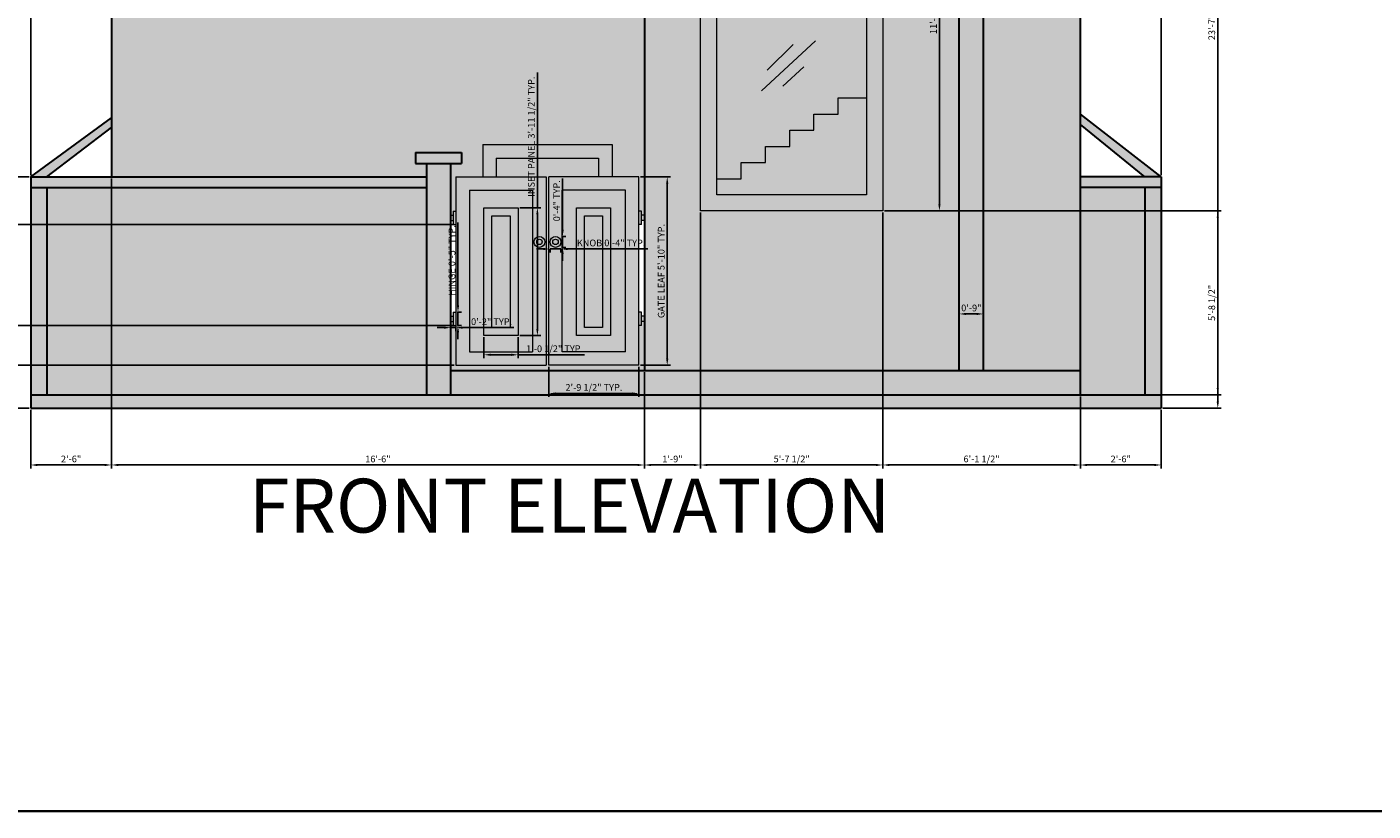
# Model space of a CAD drawing. Units: inches. Extents: x 6038 to 7543, y 3772 to 5131.
# Tile 2 of 14: x 6290 to 6790, y 3772 to 4063. Entities that reach past the tile are written whole.
import ezdxf

# ---------------------------------------------------------------- set-up
doc = ezdxf.new("R2010")
doc.units = ezdxf.units.IN
for name, color, linetype, lineweight in [('A-ANNO-DIMS', 4, 'Continuous', 18), ('A-ANNO-TITL', 3, 'Continuous', 30), ('A-ANNO-TTLB', 1, 'Continuous', 35), ('A-ELEV', 7, 'Continuous', 30), ('A-ELEV-DOOR-PATT', 209, 'Continuous', 13), ('A-ELEV-FRAM-PATT', 7, 'Continuous', 13), ('A-ELEV-GATE', 7, 'Continuous', 20), ('A-ELEV-GLAZ', 7, 'Continuous', 18), ('A-ELEV-STRS', 7, 'Continuous', 18)]:
    doc.layers.add(name, color=color, linetype=linetype, lineweight=lineweight)
for name, color, linetype, lineweight, true_color in [('A-ELEV-BASE-PATT', 253, 'Continuous', 13, 0xb4b5b6), ('A-ELEV-GLAZ-PATT', 141, 'Continuous', 13, 0xadddf7), ('A-ELEV-METL-PATT', 252, 'Continuous', 13, 0x939598), ('A-ELEV-PANL-PATT', 165, 'Continuous', 13, 0x5e67af), ('A-ELEV-TRIM-PATT', 85, 'Continuous', 13, 0x58ba48), ('A-ELEV-WALL-PATT', 11, 'Continuous', 13, 0xf27172)]:
    doc.layers.add(name, color=color, linetype=linetype, lineweight=lineweight, true_color=true_color)
doc.styles.get("Standard").update_dxf_attribs({"font": 'arial.ttf'})
doc.dimstyles.new('ISO-25', dxfattribs={"dimtxt": 2.5, "dimasz": 2.5, "dimexe": 1.25, "dimexo": 0.625, "dimtad": 1, "dimdec": 0, "dimlunit": 3, "dimtxsty": 'Standard', "dimcen": 2.5, "dimadec": 0, "dimazin": 0, "dimtfac": 1, "dimtdec": 0, "dimtmove": 0, "dimatfit": 3, "dimfxl": 1, "dimarcsym": 0})

# ---------------------------------------------------------------- blocks, each defined once
blk = doc.blocks.new('GATE-LEAF-FRAME-ELEV')
for p, q in [((0, 70), (0, 0)), ((0, 70), (33.5, 70)), ((33.5, 70), (33.5, 0)), ((5, 65), (5, 5)), ((5, 65), (28.5, 65)), ((28.5, 65), (28.5, 5)), ((5, 5), (28.5, 5)), ((0, 0), (33.5, 0))]:
    blk.add_line(p, q)
blk = doc.blocks.new('GATE-LEAF-INSET-ELEV')
for points in [[(0, 47.53), (12.73, 47.53), (12.73, 0), (0, 0)], [(3, 44.53), (9.73, 44.53), (9.73, 3), (3, 3)]]:
    blk.add_lwpolyline(points, close=True)
blk = doc.blocks.new('GATE-HINGE-ELEV')
for p, q in [((0, 3.5), (1, 3.5)), ((0, 1.5), (1, 1.5)), ((1, 5), (2, 5)), ((1, 5), (1, 0)), ((1, 0), (2, 0))]:
    blk.add_line(p, q)
blk = doc.blocks.new('GATE-KNOB-ELEV')
for radius in [2.03, 1.03]:
    blk.add_circle((2.03, 2.03), radius)
blk = doc.blocks.new('GLASS-MARK-TALL')
for p, q in [((0, 0), (20.02, 18.51)), ((2.13, 7.66), (11.71, 17.23)), ((7.88, 1.7), (15.76, 8.93))]:
    blk.add_line(p, q)
blk = doc.blocks.new('*D44')
at = {"layer": 'A-ANNO-DIMS', "color": 0, "lineweight": -2, "transparency": 16777216}
for p, q in [((6450.17, 3959.96), (6450.17, 3990.84)), ((6450.04, 3957.46), (6451.42, 3957.46)), ((6450.17, 3952.46), (6450.17, 3957.46)), ((6450.04, 3952.46), (6451.42, 3952.46)), ((6450.17, 3949.96), (6450.17, 3947.46))]:
    blk.add_line(p, q, dxfattribs=at)
at = {"layer": 'A-ANNO-DIMS', "color": 0, "transparency": 16777216}
for points in [[(6449.75, 3959.96), (6450.58, 3959.96), (6450.17, 3957.46)], [(6449.75, 3949.96), (6450.58, 3949.96), (6450.17, 3952.46)]]:
    blk.add_solid(points, dxfattribs=at)
at = {"layer": 'Defpoints', "color": 0, "transparency": 16777216}
for p in [(6449.42, 3957.46), (6450.17, 3957.46), (6449.42, 3952.46)]:
    blk.add_point(p, dxfattribs=at)
at = {"layer": 'A-ANNO-DIMS', "color": 0, "transparency": 16777216, "insert": (6448.25, 3976.65), "char_height": 2.5, "attachment_point": 5, "rotation": 90}
blk.add_mtext('HINGE 0\'-5" TYP.', dxfattribs=at)
blk = doc.blocks.new('*D45')
at = {"layer": 'A-ANNO-DIMS', "color": 0, "lineweight": -2, "transparency": 16777216}
for p, q in [((6444.92, 3951.71), (6442.42, 3951.71)), ((6447.42, 3951.83), (6447.42, 3950.46)), ((6447.42, 3951.71), (6449.42, 3951.71)), ((6449.42, 3951.83), (6449.42, 3950.46)), ((6451.92, 3951.71), (6470.91, 3951.71))]:
    blk.add_line(p, q, dxfattribs=at)
at = {"layer": 'A-ANNO-DIMS', "color": 0, "transparency": 16777216}
for points in [[(6444.92, 3952.13), (6444.92, 3951.29), (6447.42, 3951.71)], [(6451.92, 3952.13), (6451.92, 3951.29), (6449.42, 3951.71)]]:
    blk.add_solid(points, dxfattribs=at)
at = {"layer": 'Defpoints', "color": 0, "transparency": 16777216}
for p in [(6447.42, 3952.46), (6449.42, 3952.46), (6449.42, 3951.71)]:
    blk.add_point(p, dxfattribs=at)
at = {"layer": 'A-ANNO-DIMS', "color": 0, "transparency": 16777216, "insert": (6462.66, 3953.61), "char_height": 2.5, "attachment_point": 5}
blk.add_mtext('0\'-2" TYP.', dxfattribs=at)
blk = doc.blocks.new('*D46')
at = {"layer": 'A-ANNO-DIMS', "color": 0, "lineweight": -2, "transparency": 16777216}
for p, q in [((6518.04, 4007.75), (6529.17, 4007.75)), ((6527.92, 4005.25), (6527.92, 3940.25)), ((6518.04, 3937.75), (6529.17, 3937.75))]:
    blk.add_line(p, q, dxfattribs=at)
at = {"layer": 'A-ANNO-DIMS', "color": 0, "transparency": 16777216}
for points in [[(6527.5, 4005.25), (6528.33, 4005.25), (6527.92, 4007.75)], [(6527.5, 3940.25), (6528.33, 3940.25), (6527.92, 3937.75)]]:
    blk.add_solid(points, dxfattribs=at)
at = {"layer": 'Defpoints', "color": 0, "transparency": 16777216}
for p in [(6517.42, 4007.75), (6517.42, 3937.75), (6527.92, 3937.75)]:
    blk.add_point(p, dxfattribs=at)
at = {"layer": 'A-ANNO-DIMS', "color": 0, "transparency": 16777216, "insert": (6526, 3972.75), "char_height": 2.5, "attachment_point": 5, "rotation": 90}
blk.add_mtext('GATE LEAF 5\'-10" TYP.', dxfattribs=at)
blk = doc.blocks.new('*D47')
at = {"layer": 'A-ANNO-DIMS', "color": 0, "lineweight": -2, "transparency": 16777216}
for p, q in [((6483.92, 3937.12), (6483.92, 3926)), ((6517.42, 3937.12), (6517.42, 3926)), ((6514.92, 3927.25), (6486.42, 3927.25))]:
    blk.add_line(p, q, dxfattribs=at)
at = {"layer": 'A-ANNO-DIMS', "color": 0, "transparency": 16777216}
for points in [[(6486.42, 3927.66), (6486.42, 3926.83), (6483.92, 3927.25)], [(6514.92, 3927.66), (6514.92, 3926.83), (6517.42, 3927.25)]]:
    blk.add_solid(points, dxfattribs=at)
at = {"layer": 'Defpoints', "color": 0, "transparency": 16777216}
for p in [(6483.92, 3937.75), (6517.42, 3937.75), (6483.92, 3927.25)]:
    blk.add_point(p, dxfattribs=at)
at = {"layer": 'A-ANNO-DIMS', "color": 0, "transparency": 16777216, "insert": (6500.67, 3929.17), "char_height": 2.5, "attachment_point": 5}
blk.add_mtext('2\'-9 1/2" TYP.', dxfattribs=at)
blk = doc.blocks.new('*D48')
at = {"layer": 'A-ANNO-DIMS', "color": 0, "lineweight": -2, "transparency": 16777216}
for p, q in [((6479.67, 3996.29), (6479.67, 4046.54)), ((6473.17, 3996.29), (6480.92, 3996.29)), ((6479.67, 3951.26), (6479.67, 3993.79)), ((6473.17, 3948.76), (6480.92, 3948.76))]:
    blk.add_line(p, q, dxfattribs=at)
at = {"layer": 'A-ANNO-DIMS', "color": 0, "transparency": 16777216}
for points in [[(6479.25, 3993.79), (6480.09, 3993.79), (6479.67, 3996.29)], [(6479.25, 3951.26), (6480.09, 3951.26), (6479.67, 3948.76)]]:
    blk.add_solid(points, dxfattribs=at)
at = {"layer": 'Defpoints', "color": 0, "transparency": 16777216}
for p in [(6472.54, 3996.29), (6479.67, 3996.29), (6472.54, 3948.76)]:
    blk.add_point(p, dxfattribs=at)
at = {"layer": 'A-ANNO-DIMS', "color": 0, "transparency": 16777216, "insert": (6477.75, 4022.67), "char_height": 2.5, "attachment_point": 5, "rotation": 90}
blk.add_mtext('INSET PANEL 3\'-11 1/2" TYP.', dxfattribs=at)
blk = doc.blocks.new('*D49')
at = {"layer": 'A-ANNO-DIMS', "color": 0, "lineweight": -2, "transparency": 16777216}
for p, q in [((6459.81, 3948.14), (6459.81, 3940.38)), ((6472.54, 3948.14), (6472.54, 3940.38)), ((6462.31, 3941.63), (6470.04, 3941.63)), ((6472.54, 3941.63), (6497.12, 3941.63))]:
    blk.add_line(p, q, dxfattribs=at)
at = {"layer": 'A-ANNO-DIMS', "color": 0, "transparency": 16777216}
for points in [[(6462.31, 3942.05), (6462.31, 3941.22), (6459.81, 3941.63)], [(6470.04, 3942.05), (6470.04, 3941.22), (6472.54, 3941.63)]]:
    blk.add_solid(points, dxfattribs=at)
at = {"layer": 'Defpoints', "color": 0, "transparency": 16777216}
for p in [(6459.81, 3948.76), (6472.54, 3948.76), (6472.54, 3941.63)]:
    blk.add_point(p, dxfattribs=at)
at = {"layer": 'A-ANNO-DIMS', "color": 0, "transparency": 16777216, "insert": (6486.08, 3943.55), "char_height": 2.5, "attachment_point": 5}
blk.add_mtext('1\'-0 1/2" TYP.', dxfattribs=at)
blk = doc.blocks.new('*D50')
at = {"layer": 'A-ANNO-DIMS', "color": 0, "lineweight": -2, "transparency": 16777216}
for p, q in [((6481.87, 3980.94), (6479.37, 3980.94)), ((6484.37, 3980.94), (6488.44, 3980.94)), ((6484.37, 3980.92), (6484.37, 3979.69)), ((6488.44, 3980.92), (6488.44, 3979.69)), ((6490.94, 3980.94), (6520.69, 3980.94))]:
    blk.add_line(p, q, dxfattribs=at)
at = {"layer": 'A-ANNO-DIMS', "color": 0, "transparency": 16777216}
for points in [[(6481.87, 3981.35), (6481.87, 3980.52), (6484.37, 3980.94)], [(6490.94, 3981.35), (6490.94, 3980.52), (6488.44, 3980.94)]]:
    blk.add_solid(points, dxfattribs=at)
at = {"layer": 'Defpoints', "color": 0, "transparency": 16777216}
for p in [(6484.37, 3981.55), (6488.44, 3981.55), (6488.44, 3980.94)]:
    blk.add_point(p, dxfattribs=at)
at = {"layer": 'A-ANNO-DIMS', "color": 0, "transparency": 16777216, "insert": (6507.06, 3982.86), "char_height": 2.5, "attachment_point": 5}
blk.add_mtext('KNOB 0\'-4" TYP.', dxfattribs=at)
blk = doc.blocks.new('*D51')
at = {"layer": 'A-ANNO-DIMS', "color": 0, "lineweight": -2, "transparency": 16777216}
for p, q in [((6489.05, 3988.11), (6489.05, 4007.1)), ((6489.05, 3981.55), (6489.05, 3985.61)), ((6489.06, 3985.61), (6490.3, 3985.61)), ((6489.06, 3981.55), (6490.3, 3981.55)), ((6489.05, 3979.05), (6489.05, 3976.55))]:
    blk.add_line(p, q, dxfattribs=at)
at = {"layer": 'A-ANNO-DIMS', "color": 0, "transparency": 16777216}
for points in [[(6488.63, 3988.11), (6489.47, 3988.11), (6489.05, 3985.61)], [(6488.63, 3979.05), (6489.47, 3979.05), (6489.05, 3981.55)]]:
    blk.add_solid(points, dxfattribs=at)
at = {"layer": 'Defpoints', "color": 0, "transparency": 16777216}
for p in [(6488.44, 3985.61), (6488.44, 3981.55), (6489.05, 3985.61)]:
    blk.add_point(p, dxfattribs=at)
at = {"layer": 'A-ANNO-DIMS', "color": 0, "transparency": 16777216, "insert": (6487.15, 3998.86), "char_height": 2.5, "attachment_point": 5, "rotation": 90}
blk.add_mtext('0\'-4" TYP.', dxfattribs=at)
blk = doc.blocks.new('*D66')
at = {"layer": 'A-ANNO-DIMS', "color": 0, "lineweight": -2, "transparency": 16777216}
for p, q in [((6291.42, 4008.37), (6291.42, 4227.06)), ((6711.42, 4008.37), (6711.42, 4227.06)), ((6293.92, 4225.81), (6708.92, 4225.81))]:
    blk.add_line(p, q, dxfattribs=at)
at = {"layer": 'A-ANNO-DIMS', "color": 0, "transparency": 16777216}
for points in [[(6293.92, 4226.22), (6293.92, 4225.39), (6291.42, 4225.81)], [(6708.92, 4226.22), (6708.92, 4225.39), (6711.42, 4225.81)]]:
    blk.add_solid(points, dxfattribs=at)
at = {"layer": 'Defpoints', "color": 0, "transparency": 16777216}
for p in [(6711.42, 4225.81), (6291.42, 4007.75), (6711.42, 4007.75)]:
    blk.add_point(p, dxfattribs=at)
at = {"layer": 'A-ANNO-DIMS', "color": 0, "transparency": 16777216, "insert": (6501.42, 4227.71), "char_height": 2.5, "attachment_point": 5}
blk.add_mtext('35\'-0"', dxfattribs=at)
blk = doc.blocks.new('*D67')
at = {"layer": 'A-ANNO-DIMS', "color": 0, "lineweight": -2, "transparency": 16777216}
for p, q in [((6694.04, 4204.75), (6733.73, 4204.75)), ((6732.48, 3924.25), (6732.48, 4202.25)), ((6712.04, 3921.75), (6733.73, 3921.75))]:
    blk.add_line(p, q, dxfattribs=at)
at = {"layer": 'A-ANNO-DIMS', "color": 0, "transparency": 16777216}
for points in [[(6732.06, 4202.25), (6732.89, 4202.25), (6732.48, 4204.75)], [(6732.06, 3924.25), (6732.89, 3924.25), (6732.48, 3921.75)]]:
    blk.add_solid(points, dxfattribs=at)
at = {"layer": 'Defpoints', "color": 0, "transparency": 16777216}
for p in [(6693.42, 4204.75), (6732.48, 4204.75), (6711.42, 3921.75)]:
    blk.add_point(p, dxfattribs=at)
at = {"layer": 'A-ANNO-DIMS', "color": 0, "transparency": 16777216, "insert": (6730.57, 4063.25), "char_height": 2.5, "attachment_point": 5, "rotation": 90}
blk.add_mtext('23\'-7"', dxfattribs=at)
blk = doc.blocks.new('*D68')
at = {"layer": 'A-ANNO-DIMS', "color": 0, "lineweight": -2, "transparency": 16777216}
for p, q in [((6321.42, 4007.12), (6321.42, 3899.44)), ((6291.42, 3921.12), (6291.42, 3899.44)), ((6293.92, 3900.69), (6318.92, 3900.69))]:
    blk.add_line(p, q, dxfattribs=at)
at = {"layer": 'A-ANNO-DIMS', "color": 0, "transparency": 16777216}
for points in [[(6293.92, 3901.1), (6293.92, 3900.27), (6291.42, 3900.69)], [(6318.92, 3901.1), (6318.92, 3900.27), (6321.42, 3900.69)]]:
    blk.add_solid(points, dxfattribs=at)
at = {"layer": 'Defpoints', "color": 0, "transparency": 16777216}
for p in [(6321.42, 4007.75), (6291.42, 3921.75), (6321.42, 3900.69)]:
    blk.add_point(p, dxfattribs=at)
at = {"layer": 'A-ANNO-DIMS', "color": 0, "transparency": 16777216, "insert": (6306.42, 3902.59), "char_height": 2.5, "attachment_point": 5}
blk.add_mtext('2\'-6"', dxfattribs=at)
blk = doc.blocks.new('*D69')
at = {"layer": 'A-ANNO-DIMS', "color": 0, "lineweight": -2, "transparency": 16777216}
for p, q in [((6321.42, 4007.12), (6321.42, 3899.44)), ((6519.42, 3935.12), (6519.42, 3899.44)), ((6323.92, 3900.69), (6516.92, 3900.69))]:
    blk.add_line(p, q, dxfattribs=at)
at = {"layer": 'A-ANNO-DIMS', "color": 0, "transparency": 16777216}
for points in [[(6323.92, 3901.1), (6323.92, 3900.27), (6321.42, 3900.69)], [(6516.92, 3901.1), (6516.92, 3900.27), (6519.42, 3900.69)]]:
    blk.add_solid(points, dxfattribs=at)
at = {"layer": 'Defpoints', "color": 0, "transparency": 16777216}
for p in [(6321.42, 4007.75), (6519.42, 3935.75), (6519.42, 3900.69)]:
    blk.add_point(p, dxfattribs=at)
at = {"layer": 'A-ANNO-DIMS', "color": 0, "transparency": 16777216, "insert": (6420.42, 3902.59), "char_height": 2.5, "attachment_point": 5}
blk.add_mtext('16\'-6"', dxfattribs=at)
blk = doc.blocks.new('*D70')
at = {"layer": 'A-ANNO-DIMS', "color": 0, "lineweight": -2, "transparency": 16777216}
for p, q in [((6540.32, 3994.44), (6540.32, 3899.44)), ((6519.42, 3935.12), (6519.42, 3899.44)), ((6521.92, 3900.69), (6537.82, 3900.69))]:
    blk.add_line(p, q, dxfattribs=at)
at = {"layer": 'A-ANNO-DIMS', "color": 0, "transparency": 16777216}
for points in [[(6521.92, 3901.1), (6521.92, 3900.27), (6519.42, 3900.69)], [(6537.82, 3901.1), (6537.82, 3900.27), (6540.32, 3900.69)]]:
    blk.add_solid(points, dxfattribs=at)
at = {"layer": 'Defpoints', "color": 0, "transparency": 16777216}
for p in [(6540.32, 3995.07), (6519.42, 3935.75), (6540.32, 3900.69)]:
    blk.add_point(p, dxfattribs=at)
at = {"layer": 'A-ANNO-DIMS', "color": 0, "transparency": 16777216, "insert": (6529.87, 3902.59), "char_height": 2.5, "attachment_point": 5}
blk.add_mtext('1\'-9"', dxfattribs=at)
blk = doc.blocks.new('*D71')
at = {"layer": 'A-ANNO-DIMS', "color": 0, "lineweight": -2, "transparency": 16777216}
for p, q in [((6540.32, 3994.44), (6540.32, 3899.44)), ((6607.99, 3994.44), (6607.99, 3899.44)), ((6542.82, 3900.69), (6605.49, 3900.69))]:
    blk.add_line(p, q, dxfattribs=at)
at = {"layer": 'A-ANNO-DIMS', "color": 0, "transparency": 16777216}
for points in [[(6542.82, 3901.1), (6542.82, 3900.27), (6540.32, 3900.69)], [(6605.49, 3901.1), (6605.49, 3900.27), (6607.99, 3900.69)]]:
    blk.add_solid(points, dxfattribs=at)
at = {"layer": 'Defpoints', "color": 0, "transparency": 16777216}
for p in [(6540.32, 3995.07), (6607.99, 3995.07), (6607.99, 3900.69)]:
    blk.add_point(p, dxfattribs=at)
at = {"layer": 'A-ANNO-DIMS', "color": 0, "transparency": 16777216, "insert": (6574.16, 3902.61), "char_height": 2.5, "attachment_point": 5}
blk.add_mtext('5\'-7 1/2"', dxfattribs=at)
blk = doc.blocks.new('*D72')
at = {"layer": 'A-ANNO-DIMS', "color": 0, "lineweight": -2, "transparency": 16777216}
for p, q in [((6607.99, 3994.44), (6607.99, 3899.44)), ((6681.42, 3926.12), (6681.42, 3899.44)), ((6610.49, 3900.69), (6678.92, 3900.69))]:
    blk.add_line(p, q, dxfattribs=at)
at = {"layer": 'A-ANNO-DIMS', "color": 0, "transparency": 16777216}
for points in [[(6610.49, 3901.1), (6610.49, 3900.27), (6607.99, 3900.69)], [(6678.92, 3901.1), (6678.92, 3900.27), (6681.42, 3900.69)]]:
    blk.add_solid(points, dxfattribs=at)
at = {"layer": 'Defpoints', "color": 0, "transparency": 16777216}
for p in [(6607.99, 3995.07), (6681.42, 3926.75), (6681.42, 3900.69)]:
    blk.add_point(p, dxfattribs=at)
at = {"layer": 'A-ANNO-DIMS', "color": 0, "transparency": 16777216, "insert": (6644.71, 3902.61), "char_height": 2.5, "attachment_point": 5}
blk.add_mtext('6\'-1 1/2"', dxfattribs=at)
blk = doc.blocks.new('*D73')
at = {"layer": 'A-ANNO-DIMS', "color": 0, "lineweight": -2, "transparency": 16777216}
for p, q in [((6681.42, 3926.12), (6681.42, 3899.44)), ((6711.42, 3921.12), (6711.42, 3899.44)), ((6683.92, 3900.69), (6708.92, 3900.69))]:
    blk.add_line(p, q, dxfattribs=at)
at = {"layer": 'A-ANNO-DIMS', "color": 0, "transparency": 16777216}
for points in [[(6683.92, 3901.1), (6683.92, 3900.27), (6681.42, 3900.69)], [(6708.92, 3901.1), (6708.92, 3900.27), (6711.42, 3900.69)]]:
    blk.add_solid(points, dxfattribs=at)
at = {"layer": 'Defpoints', "color": 0, "transparency": 16777216}
for p in [(6681.42, 3926.75), (6711.42, 3921.75), (6711.42, 3900.69)]:
    blk.add_point(p, dxfattribs=at)
at = {"layer": 'A-ANNO-DIMS', "color": 0, "transparency": 16777216, "insert": (6696.42, 3902.59), "char_height": 2.5, "attachment_point": 5}
blk.add_mtext('2\'-6"', dxfattribs=at)
blk = doc.blocks.new('*D74')
at = {"layer": 'A-ANNO-DIMS', "color": 0, "lineweight": -2, "transparency": 16777216}
for p, q in [((6290.79, 4007.75), (6269.11, 4007.75)), ((6270.36, 3924.25), (6270.36, 4005.25)), ((6290.79, 3921.75), (6269.11, 3921.75))]:
    blk.add_line(p, q, dxfattribs=at)
at = {"layer": 'A-ANNO-DIMS', "color": 0, "transparency": 16777216}
for points in [[(6269.94, 4005.25), (6270.77, 4005.25), (6270.36, 4007.75)], [(6269.94, 3924.25), (6270.77, 3924.25), (6270.36, 3921.75)]]:
    blk.add_solid(points, dxfattribs=at)
at = {"layer": 'Defpoints', "color": 0, "transparency": 16777216}
for p in [(6270.36, 4007.75), (6291.42, 4007.75), (6291.42, 3921.75)]:
    blk.add_point(p, dxfattribs=at)
at = {"layer": 'A-ANNO-DIMS', "color": 0, "transparency": 16777216, "insert": (6268.48, 3964.75), "char_height": 2.5, "attachment_point": 5, "rotation": 90}
blk.add_mtext('7\'-2"', dxfattribs=at)
blk = doc.blocks.new('*D75')
at = {"layer": 'A-ANNO-DIMS', "color": 0, "lineweight": -2, "transparency": 16777216}
for p, q in [((6308.79, 4097.75), (6269.11, 4097.75)), ((6270.36, 4010.25), (6270.36, 4095.25)), ((6290.79, 4007.75), (6269.11, 4007.75))]:
    blk.add_line(p, q, dxfattribs=at)
at = {"layer": 'A-ANNO-DIMS', "color": 0, "transparency": 16777216}
for points in [[(6269.94, 4095.25), (6270.77, 4095.25), (6270.36, 4097.75)], [(6269.94, 4010.25), (6270.77, 4010.25), (6270.36, 4007.75)]]:
    blk.add_solid(points, dxfattribs=at)
at = {"layer": 'Defpoints', "color": 0, "transparency": 16777216}
for p in [(6270.36, 4097.75), (6309.42, 4097.75), (6291.42, 4007.75)]:
    blk.add_point(p, dxfattribs=at)
at = {"layer": 'A-ANNO-DIMS', "color": 0, "transparency": 16777216, "insert": (6268.46, 4052.75), "char_height": 2.5, "attachment_point": 5, "rotation": 90}
blk.add_mtext('7\'-6"', dxfattribs=at)
blk = doc.blocks.new('*D77')
at = {"layer": 'A-ANNO-DIMS', "color": 0, "lineweight": -2, "transparency": 16777216}
for p, q in [((6608.62, 4137.88), (6630.3, 4137.88)), ((6629.05, 4135.38), (6629.05, 3997.57)), ((6608.62, 3995.07), (6630.3, 3995.07))]:
    blk.add_line(p, q, dxfattribs=at)
at = {"layer": 'A-ANNO-DIMS', "color": 0, "transparency": 16777216}
for points in [[(6628.64, 4135.38), (6629.47, 4135.38), (6629.05, 4137.88)], [(6628.64, 3997.57), (6629.47, 3997.57), (6629.05, 3995.07)]]:
    blk.add_solid(points, dxfattribs=at)
at = {"layer": 'Defpoints', "color": 0, "transparency": 16777216}
for p in [(6607.99, 4137.88), (6607.99, 3995.07), (6629.05, 3995.07)]:
    blk.add_point(p, dxfattribs=at)
at = {"layer": 'A-ANNO-DIMS', "color": 0, "transparency": 16777216, "insert": (6627.17, 4066.47), "char_height": 2.5, "attachment_point": 5, "rotation": 90}
blk.add_mtext('11\'-11"', dxfattribs=at)
blk = doc.blocks.new('*D78')
at = {"layer": 'A-ANNO-DIMS', "color": 0, "lineweight": -2, "transparency": 16777216}
for p, q in [((6608.62, 3995.07), (6733.73, 3995.07)), ((6732.48, 3929.25), (6732.48, 3992.57)), ((6682.04, 3926.75), (6733.73, 3926.75))]:
    blk.add_line(p, q, dxfattribs=at)
at = {"layer": 'A-ANNO-DIMS', "color": 0, "transparency": 16777216}
for points in [[(6732.06, 3992.57), (6732.89, 3992.57), (6732.48, 3995.07)], [(6732.06, 3929.25), (6732.89, 3929.25), (6732.48, 3926.75)]]:
    blk.add_solid(points, dxfattribs=at)
at = {"layer": 'Defpoints', "color": 0, "transparency": 16777216}
for p in [(6607.99, 3995.07), (6732.48, 3995.07), (6681.42, 3926.75)]:
    blk.add_point(p, dxfattribs=at)
at = {"layer": 'A-ANNO-DIMS', "color": 0, "transparency": 16777216, "insert": (6730.56, 3960.91), "char_height": 2.5, "attachment_point": 5, "rotation": 90}
blk.add_mtext('5\'-8 1/2"', dxfattribs=at)
blk = doc.blocks.new('*D82')
at = {"layer": 'A-ANNO-DIMS', "color": 0, "lineweight": -2, "transparency": 16777216}
for p, q in [((6636.42, 3936.37), (6636.42, 3958.06)), ((6638.92, 3956.81), (6642.92, 3956.81)), ((6645.42, 3936.37), (6645.42, 3958.06))]:
    blk.add_line(p, q, dxfattribs=at)
at = {"layer": 'A-ANNO-DIMS', "color": 0, "transparency": 16777216}
for points in [[(6638.92, 3957.22), (6638.92, 3956.39), (6636.42, 3956.81)], [(6642.92, 3957.22), (6642.92, 3956.39), (6645.42, 3956.81)]]:
    blk.add_solid(points, dxfattribs=at)
at = {"layer": 'Defpoints', "color": 0, "transparency": 16777216}
for p in [(6645.42, 3956.81), (6636.42, 3935.75), (6645.42, 3935.75)]:
    blk.add_point(p, dxfattribs=at)
at = {"layer": 'A-ANNO-DIMS', "color": 0, "transparency": 16777216, "insert": (6640.92, 3958.71), "char_height": 2.5, "attachment_point": 5}
blk.add_mtext('0\'-9"', dxfattribs=at)
blk = doc.blocks.new('*D83')
at = {"layer": 'A-ANNO-DIMS', "color": 0, "lineweight": -2, "transparency": 16777216}
for p, q in [((6448.79, 3952.46), (6269.11, 3952.46)), ((6270.36, 3940.25), (6270.36, 3949.96)), ((6448.79, 3937.75), (6269.11, 3937.75))]:
    blk.add_line(p, q, dxfattribs=at)
at = {"layer": 'A-ANNO-DIMS', "color": 0, "transparency": 16777216}
for points in [[(6269.94, 3949.96), (6270.77, 3949.96), (6270.36, 3952.46)], [(6269.94, 3940.25), (6270.77, 3940.25), (6270.36, 3937.75)]]:
    blk.add_solid(points, dxfattribs=at)
at = {"layer": 'Defpoints', "color": 0, "transparency": 16777216}
for p in [(6270.36, 3952.46), (6449.42, 3952.46), (6449.42, 3937.75)]:
    blk.add_point(p, dxfattribs=at)
at = {"layer": 'A-ANNO-DIMS', "color": 0, "transparency": 16777216, "insert": (6268.44, 3945.1), "char_height": 2.5, "attachment_point": 5, "rotation": 90}
blk.add_mtext('1\'-2 1/2"', dxfattribs=at)
blk = doc.blocks.new('*D84')
at = {"layer": 'A-ANNO-DIMS', "color": 0, "lineweight": -2, "transparency": 16777216}
for p, q in [((6448.79, 3990.02), (6269.11, 3990.02)), ((6270.36, 3954.96), (6270.36, 3987.52)), ((6448.79, 3952.46), (6269.11, 3952.46))]:
    blk.add_line(p, q, dxfattribs=at)
at = {"layer": 'A-ANNO-DIMS', "color": 0, "transparency": 16777216}
for points in [[(6269.94, 3987.52), (6270.77, 3987.52), (6270.36, 3990.02)], [(6269.94, 3954.96), (6270.77, 3954.96), (6270.36, 3952.46)]]:
    blk.add_solid(points, dxfattribs=at)
at = {"layer": 'Defpoints', "color": 0, "transparency": 16777216}
for p in [(6270.36, 3990.02), (6449.42, 3990.02), (6449.42, 3952.46)]:
    blk.add_point(p, dxfattribs=at)
at = {"layer": 'A-ANNO-DIMS', "color": 0, "transparency": 16777216, "insert": (6268.44, 3971.24), "char_height": 2.5, "attachment_point": 5, "rotation": 90}
blk.add_mtext('3\'-1 1/2"', dxfattribs=at)

msp = doc.modelspace()

# ---------------------------------------------------------------- hatches: boundary and pattern name
at = {"layer": 'A-ELEV-BASE-PATT'}
h = msp.add_hatch(color=256, dxfattribs=at)
h.dxf.hatch_style = 1
h.paths.add_polyline_path([(6681.42, 3935.75), (6447.42, 3935.75), (6447.42, 3926.75), (6681.42, 3926.75)])
h = msp.add_hatch(color=256, dxfattribs=at)
h.dxf.hatch_style = 1
h.paths.add_polyline_path([(6711.42, 3926.75), (6291.42, 3926.75), (6291.42, 3921.75), (6711.42, 3921.75)])
at = {"layer": 'A-ELEV-DOOR-PATT'}
h = msp.add_hatch(color=256, dxfattribs=at)
h.dxf.hatch_style = 1
h.paths.add_polyline_path([(6507.42, 4019.75), (6459.42, 4019.75), (6459.42, 4007.75), (6464.42, 4007.75), (6464.42, 4014.75), (6502.42, 4014.75), (6502.42, 4007.75), (6507.42, 4007.75)])
h = msp.add_hatch(color=256, dxfattribs=at)
h.dxf.hatch_style = 1
h.paths.add_polyline_path([(6502.42, 4014.75), (6464.42, 4014.75), (6464.42, 4007.75), (6482.92, 4007.75), (6482.92, 3937.75), (6449.42, 3937.75), (6449.42, 3952.46), (6448.42, 3952.46), (6448.42, 3953.96), (6447.42, 3953.96), (6447.42, 3935.75), (6519.42, 3935.75), (6519.42, 3953.96), (6518.42, 3953.96), (6518.42, 3952.46), (6517.42, 3952.46), (6517.42, 3937.75), (6483.92, 3937.75), (6483.92, 4007.75), (6502.42, 4007.75)])
at = {"layer": 'A-ELEV-FRAM-PATT'}
h = msp.add_hatch(color=256, dxfattribs=at)
h.dxf.hatch_style = 1
h.paths.add_polyline_path([(6607.99, 4137.88), (6540.32, 4137.88), (6540.32, 3995.07), (6607.99, 3995.07)])
h.paths.add_polyline_path([(6546.32, 4131.88), (6601.99, 4131.88), (6601.99, 4001.07), (6546.32, 4001.07), (6546.32, 4007.07)], flags=16)
h = msp.add_hatch(color=256, dxfattribs=at)
h.dxf.hatch_style = 1
h.paths.add_polyline_path([(6482.92, 4007.75), (6449.42, 4007.75), (6449.42, 3937.75), (6482.92, 3937.75)])
h.paths.add_polyline_path([(6454.42, 4002.75), (6477.92, 4002.75), (6477.92, 3942.75), (6454.42, 3942.75)], flags=16)
h.paths.add_polyline_path([(6459.81, 3996.29), (6472.54, 3996.29), (6472.54, 3948.76), (6459.81, 3948.76)], flags=0)
h.paths.add_polyline_path([(6462.81, 3993.29), (6469.54, 3993.29), (6469.54, 3951.76), (6462.81, 3951.76)], flags=0)
h.paths.add_polyline_path([(6482.48, 3983.58, -1), (6478.41, 3983.58, -1)], flags=16)
h.paths.add_polyline_path([(6481.48, 3983.58, -1), (6479.41, 3983.58, -1)], flags=0)
h.paths.add_polyline_path([(6472.54, 3996.29), (6459.81, 3996.29), (6459.81, 3948.76), (6472.54, 3948.76)], flags=0)
h.paths.add_polyline_path([(6449.42, 3995.02), (6448.42, 3995.02), (6448.42, 3990.02), (6449.42, 3990.02)])
h.paths.add_polyline_path([(6448.42, 3993.52), (6447.42, 3993.52), (6447.42, 3991.52), (6448.42, 3991.52)])
h.paths.add_polyline_path([(6517.42, 4007.75), (6483.92, 4007.75), (6483.92, 3937.75), (6517.42, 3937.75)])
h.paths.add_polyline_path([(6488.92, 4002.75), (6512.42, 4002.75), (6512.42, 3942.75), (6488.92, 3942.75)], flags=16)
h.paths.add_polyline_path([(6494.15, 3996.29), (6506.88, 3996.29), (6506.88, 3948.76), (6494.15, 3948.76)], flags=0)
h.paths.add_polyline_path([(6497.15, 3993.29), (6503.88, 3993.29), (6503.88, 3951.76), (6497.15, 3951.76)], flags=0)
h.paths.add_polyline_path([(6488.44, 3983.58, -1), (6484.37, 3983.58, -1)], flags=16)
h.paths.add_polyline_path([(6487.44, 3983.58, -1), (6485.37, 3983.58, -1)], flags=0)
h.paths.add_polyline_path([(6518.42, 3995.02), (6517.42, 3995.02), (6517.42, 3990.02), (6518.42, 3990.02)])
h.paths.add_polyline_path([(6519.42, 3993.52), (6518.42, 3993.52), (6518.42, 3991.52), (6519.42, 3991.52)])
h.paths.add_polyline_path([(6518.42, 3957.46), (6517.42, 3957.46), (6517.42, 3952.46), (6518.42, 3952.46)])
h.paths.add_polyline_path([(6519.42, 3955.96), (6518.42, 3955.96), (6518.42, 3953.96), (6519.42, 3953.96)])
h.paths.add_polyline_path([(6449.42, 3957.46), (6448.42, 3957.46), (6448.42, 3952.46), (6449.42, 3952.46)])
h.paths.add_polyline_path([(6448.42, 3955.96), (6447.42, 3955.96), (6447.42, 3953.96), (6448.42, 3953.96)])
h = msp.add_hatch(color=256, dxfattribs=at)
h.dxf.hatch_style = 1
h.paths.add_polyline_path([(6472.54, 3996.29), (6459.81, 3996.29), (6459.81, 3948.76), (6472.54, 3948.76)])
h.paths.add_polyline_path([(6462.81, 3993.29), (6469.54, 3993.29), (6469.54, 3951.76), (6462.81, 3951.76)], flags=16)
h.paths.add_polyline_path([(6506.88, 3996.29), (6494.15, 3996.29), (6494.15, 3948.76), (6506.88, 3948.76)])
h.paths.add_polyline_path([(6497.15, 3993.29), (6503.88, 3993.29), (6503.88, 3951.76), (6497.15, 3951.76)], flags=16)
at = {"layer": 'A-ELEV-GLAZ-PATT'}
h = msp.add_hatch(color=256, dxfattribs=at)
h.dxf.hatch_style = 1
h.paths.add_polyline_path([(6601.99, 4131.88), (6546.32, 4131.88), (6546.32, 4007.07), (6555.42, 4007.07), (6555.42, 4013.07), (6564.42, 4013.07), (6564.42, 4019.07), (6573.42, 4019.07), (6573.42, 4025.07), (6582.42, 4025.07), (6582.42, 4031.07), (6591.42, 4031.07), (6591.42, 4037.07), (6601.99, 4037.07)])
h.paths.add_polyline_path([(6601.99, 4037.07), (6591.42, 4037.07), (6591.42, 4031.07), (6582.42, 4031.07), (6582.42, 4025.07), (6573.42, 4025.07), (6573.42, 4019.07), (6564.42, 4019.07), (6564.42, 4013.07), (6555.42, 4013.07), (6555.42, 4007.07), (6546.32, 4007.07), (6546.32, 4001.07), (6601.99, 4001.07)])
h.paths.add_polyline_path([(6519.42, 4135.75), (6330.42, 4135.75), (6330.42, 4103.75), (6519.42, 4103.75)])
at = {"layer": 'A-ELEV-METL-PATT'}
h = msp.add_hatch(color=256, dxfattribs=at)
h.dxf.hatch_style = 1
h.paths.add_polyline_path([(6519.42, 4139.75), (6330.42, 4139.75), (6330.42, 4135.75), (6519.42, 4135.75)])
h.paths.add_polyline_path([(6519.42, 4103.75), (6330.42, 4103.75), (6330.42, 4099.75), (6519.42, 4099.75)])
h.paths.add_polyline_path([(6469.54, 3993.29), (6462.81, 3993.29), (6462.81, 3951.76), (6469.54, 3951.76)], flags=0)
h.paths.add_polyline_path([(6477.92, 4002.75), (6454.42, 4002.75), (6454.42, 3942.75), (6477.92, 3942.75)])
h.paths.add_polyline_path([(6459.81, 3996.29), (6472.54, 3996.29), (6472.54, 3948.76), (6459.81, 3948.76)], flags=16)
h.paths.add_polyline_path([(6462.81, 3993.29), (6469.54, 3993.29), (6469.54, 3951.76), (6462.81, 3951.76)], flags=0)
h.paths.add_polyline_path([(6503.88, 3993.29), (6497.15, 3993.29), (6497.15, 3951.76), (6503.88, 3951.76)], flags=0)
h.paths.add_polyline_path([(6512.42, 4002.75), (6488.92, 4002.75), (6488.92, 3942.75), (6512.42, 3942.75)])
h.paths.add_polyline_path([(6506.88, 3948.76), (6494.15, 3948.76), (6494.15, 3996.29), (6506.88, 3996.29)], flags=16)
h.paths.add_polyline_path([(6503.88, 3951.76), (6497.15, 3951.76), (6497.15, 3993.29), (6503.88, 3993.29)], flags=0)
h = msp.add_hatch(color=256, dxfattribs=at)
h.dxf.hatch_style = 1
h.paths.add_polyline_path([(6469.54, 3993.29), (6462.81, 3993.29), (6462.81, 3951.76), (6469.54, 3951.76)])
h.paths.add_polyline_path([(6503.88, 3993.29), (6497.15, 3993.29), (6497.15, 3951.76), (6503.88, 3951.76)])
h = msp.add_hatch(color=256, dxfattribs=at)
h.dxf.hatch_style = 1
h.paths.add_polyline_path([(6478.41, 3983.58, 1), (6482.48, 3983.58, 1)])
h.paths.add_polyline_path([(6481.48, 3983.58, -1), (6479.41, 3983.58, -1)], flags=16)
h.paths.add_polyline_path([(6484.37, 3983.58, 1), (6488.44, 3983.58, 1)])
h.paths.add_polyline_path([(6487.44, 3983.58, -1), (6485.37, 3983.58, -1)], flags=16)
h = msp.add_hatch(color=256, dxfattribs=at)
h.dxf.hatch_style = 1
h.paths.add_polyline_path([(6479.41, 3983.58, 1), (6481.48, 3983.58, 1)])
h.paths.add_polyline_path([(6485.37, 3983.58, 1), (6487.44, 3983.58, 1)])
at = {"layer": 'A-ELEV-PANL-PATT'}
h = msp.add_hatch(color=256, dxfattribs=at)
h.dxf.hatch_style = 1
h.paths.add_polyline_path([(6438.42, 4003.75), (6297.42, 4003.75), (6297.42, 3926.75), (6438.42, 3926.75)])
h.paths.add_polyline_path([(6705.42, 4003.75), (6681.42, 4003.75), (6681.42, 3926.75), (6705.42, 3926.75)])
h.paths.add_polyline_path([(6711.42, 4003.75), (6705.42, 4003.75), (6705.42, 3926.75), (6711.42, 3926.75)])
h.paths.add_polyline_path([(6297.42, 4003.75), (6291.42, 4003.75), (6291.42, 3926.75), (6297.42, 3926.75)])
h.paths.add_polyline_path([(6330.42, 4199.75), (6321.42, 4199.75), (6321.42, 4097.75), (6330.42, 4097.75)])
h.paths.add_polyline_path([(6636.42, 4166.75), (6519.42, 4166.75), (6519.42, 3935.75), (6636.42, 3935.75)])
h.paths.add_polyline_path([(6607.99, 3995.07), (6540.32, 3995.07), (6540.32, 4137.88), (6607.99, 4137.88)], flags=16)
h.paths.add_polyline_path([(6601.99, 4001.07), (6546.32, 4001.07), (6546.32, 4007.07), (6546.32, 4131.88), (6601.99, 4131.88)], flags=0)
at = {"layer": 'A-ELEV-TRIM-PATT'}
h = msp.add_hatch(color=256, dxfattribs=at)
h.dxf.hatch_style = 1
h.paths.add_polyline_path([(6645.42, 4175.75), (6519.42, 4175.75), (6519.42, 4166.75), (6636.42, 4166.75), (6636.42, 3935.75), (6645.42, 3935.75)])
h.paths.add_polyline_path([(6519.42, 4097.75), (6309.42, 4097.75), (6309.42, 4091.75), (6519.42, 4091.75)])
h.paths.add_polyline_path([(6693.42, 4097.75), (6681.42, 4097.75), (6681.42, 4091.75), (6693.42, 4091.75)])
h.paths.add_polyline_path([(6693.42, 4204.75), (6309.42, 4204.75), (6309.42, 4199.75), (6693.42, 4199.75)])
h.paths.add_polyline_path([(6438.42, 4007.75), (6291.42, 4007.75), (6291.42, 4003.75), (6438.42, 4003.75)])
h.paths.add_polyline_path([(6321.42, 4026.12), (6321.42, 4029.67), (6291.42, 4007.75), (6297.42, 4007.75)])
h.paths.add_polyline_path([(6681.42, 4031.03), (6681.42, 4027.16), (6705.42, 4007.75), (6711.42, 4007.75)])
h.paths.add_polyline_path([(6711.42, 4007.75), (6681.42, 4007.75), (6681.42, 4003.75), (6711.42, 4003.75)])
h.paths.add_polyline_path([(6451.42, 4016.75), (6434.42, 4016.75), (6434.42, 4012.75), (6451.42, 4012.75)])
at = {"layer": 'A-ELEV-WALL-PATT'}
h = msp.add_hatch(color=256, dxfattribs=at)
h.dxf.hatch_style = 1
h.paths.add_polyline_path([(6519.42, 4091.75), (6321.42, 4091.75), (6321.42, 4007.75), (6438.42, 4007.75), (6438.42, 4012.75), (6434.42, 4012.75), (6434.42, 4016.75), (6451.42, 4016.75), (6451.42, 4012.75), (6447.42, 4012.75), (6447.42, 3993.52), (6448.42, 3993.52), (6448.42, 3995.02), (6449.42, 3995.02), (6449.42, 4007.75), (6459.42, 4007.75), (6459.42, 4019.75), (6507.42, 4019.75), (6507.42, 4007.75), (6517.42, 4007.75), (6517.42, 3995.02), (6518.42, 3995.02), (6518.42, 3993.52), (6519.42, 3993.52)])
h.paths.add_polyline_path([(6681.42, 4199.75), (6519.42, 4199.75), (6519.42, 4175.75), (6645.42, 4175.75), (6645.42, 3935.75), (6681.42, 3935.75)])
h = msp.add_hatch(color=256, dxfattribs=at)
h.dxf.hatch_style = 1
h.paths.add_polyline_path([(6447.42, 4012.75), (6438.42, 4012.75), (6438.42, 3926.75), (6447.42, 3926.75)])

# ---------------------------------------------------------------- linework, layer by layer
at = {"layer": 'A-ANNO-TTLB'}
msp.add_lwpolyline([(6037.83, 5130.86), (7542.53, 5130.86), (7542.53, 3772.09), (6037.83, 3772.09)], close=True, dxfattribs=at)
at = {"layer": 'A-ELEV'}
for p, q in [((6519.42, 4199.75), (6519.42, 3935.75)), ((6681.42, 3926.75), (6681.42, 4199.75)), ((6645.42, 3935.75), (6645.42, 4175.75)), ((6636.42, 3935.75), (6636.42, 4166.75)), ((6321.42, 4091.75), (6321.42, 4007.75)), ((6291.42, 4007.75), (6321.42, 4029.67)), ((6711.42, 4007.75), (6681.42, 4031.03)), ((6705.42, 4007.75), (6681.42, 4027.16)), ((6297.42, 4007.75), (6321.42, 4026.12)), ((6434.42, 4016.75), (6451.42, 4016.75)), ((6434.42, 4016.75), (6434.42, 4012.75)), ((6451.42, 4016.75), (6451.42, 4012.75)), ((6434.42, 4012.75), (6451.42, 4012.75)), ((6438.42, 4012.75), (6438.42, 3926.75)), ((6447.42, 4012.75), (6447.42, 3926.75)), ((6291.42, 4007.75), (6438.42, 4007.75)), ((6291.42, 4007.75), (6291.42, 3921.75)), ((6711.42, 4007.75), (6681.42, 4007.75)), ((6711.42, 4007.75), (6711.42, 3921.75)), ((6291.42, 4003.75), (6438.42, 4003.75)), ((6297.42, 4003.75), (6297.42, 3926.75)), ((6711.42, 4003.75), (6681.42, 4003.75)), ((6705.42, 4003.75), (6705.42, 3926.75)), ((6447.42, 3935.75), (6681.42, 3935.75)), ((6291.42, 3926.75), (6711.42, 3926.75)), ((6291.42, 3921.75), (6711.42, 3921.75))]:
    msp.add_line(p, q, dxfattribs=at)
at = {"layer": 'A-ELEV-GATE'}
for p, q in [((6459.42, 4019.75), (6459.42, 4007.75)), ((6459.42, 4019.75), (6507.42, 4019.75)), ((6507.42, 4019.75), (6507.42, 4007.75)), ((6464.42, 4014.75), (6502.42, 4014.75)), ((6464.42, 4014.75), (6464.42, 4007.75)), ((6502.42, 4014.75), (6502.42, 4007.75))]:
    msp.add_line(p, q, dxfattribs=at)
at = {"layer": 'A-ELEV-GLAZ'}
for points in [[(6540.32, 4137.88), (6607.99, 4137.88), (6607.99, 3995.07), (6540.32, 3995.07)], [(6546.32, 4131.88), (6601.99, 4131.88), (6601.99, 4001.07), (6546.32, 4001.07)]]:
    msp.add_lwpolyline(points, close=True, dxfattribs=at)
at = {"layer": 'A-ELEV-STRS'}
for p, q in [((6591.42, 4031.07), (6591.42, 4037.07)), ((6591.42, 4037.07), (6601.99, 4037.07)), ((6582.42, 4025.07), (6582.42, 4031.07)), ((6582.42, 4031.07), (6591.42, 4031.07)), ((6573.42, 4019.07), (6573.42, 4025.07)), ((6573.42, 4025.07), (6582.42, 4025.07)), ((6564.42, 4013.07), (6564.42, 4019.07)), ((6564.42, 4019.07), (6573.42, 4019.07)), ((6555.42, 4007.07), (6555.42, 4013.07)), ((6555.42, 4013.07), (6564.42, 4013.07)), ((6546.32, 4001.07), (6546.32, 4007.07)), ((6546.32, 4007.07), (6555.42, 4007.07))]:
    msp.add_line(p, q, dxfattribs=at)

# ---------------------------------------------------------------- block references
at = {"layer": 'A-ELEV-GATE'}
for name, p in [('GATE-LEAF-FRAME-ELEV', (6449.42, 3937.75)), ('GATE-HINGE-ELEV', (6447.42, 3990.02)), ('GATE-LEAF-INSET-ELEV', (6459.81, 3948.76)), ('GATE-LEAF-INSET-ELEV', (6494.15, 3948.76)), ('GATE-KNOB-ELEV', (6478.41, 3981.55)), ('GATE-KNOB-ELEV', (6484.37, 3981.55)), ('GATE-HINGE-ELEV', (6447.42, 3952.46))]:
    msp.add_blockref(name, p, dxfattribs=at)
at = {"layer": 'A-ELEV-GATE', "rotation": 180}
for name, p in [('GATE-LEAF-FRAME-ELEV', (6517.42, 4007.75)), ('GATE-HINGE-ELEV', (6519.42, 3995.02)), ('GATE-HINGE-ELEV', (6519.42, 3957.46))]:
    msp.add_blockref(name, p, dxfattribs=at)
at = {"layer": 'A-ELEV-GLAZ'}
msp.add_blockref('GLASS-MARK-TALL', (6562.95, 4039.74), dxfattribs=at)

# ---------------------------------------------------------------- texts
at = {"layer": 'A-ANNO-TITL', "insert": (6372.45, 3895.58), "char_height": 20, "attachment_point": 1}
msp.add_mtext_dynamic_manual_height_columns('FRONT ELEVATION', width=549.9641, gutter_width=12.5, heights=[0], dxfattribs=at)

# ---------------------------------------------------------------- dimensions: what is measured, and where the dimension line sits
at = {"layer": 'A-ANNO-DIMS'}
for base, p1, p2, picture, middle in [((6711.42, 4225.81), (6291.42, 4007.75), (6711.42, 4007.75), '*D66', (6501.42, 4227.71)), ((6321.42, 3900.69), (6291.42, 3921.75), (6321.42, 4007.75), '*D68', (6306.42, 3902.59)), ((6519.42, 3900.69), (6321.42, 4007.75), (6519.42, 3935.75), '*D69', (6420.42, 3902.59)), ((6540.32, 3900.69), (6519.42, 3935.75), (6540.32, 3995.07), '*D70', (6529.87, 3902.59)), ((6607.99, 3900.69), (6540.32, 3995.07), (6607.99, 3995.07), '*D71', (6574.16, 3902.61)), ((6681.42, 3900.69), (6607.99, 3995.07), (6681.42, 3926.75), '*D72', (6644.71, 3902.61)), ((6645.42, 3956.81), (6636.42, 3935.75), (6645.42, 3935.75), '*D82', (6640.92, 3958.71)), ((6711.42, 3900.69), (6681.42, 3926.75), (6711.42, 3921.75), '*D73', (6696.42, 3902.59))]:
    dim = msp.add_linear_dim(base=base, p1=p1, p2=p2, dimstyle='ISO-25', override={"dimdec": 1, "dimlfac": 1, "dimrnd": 0, "dimzin": 1, "dimdsep": 46, "dimlunit": 4, "dimfrac": 2}, dxfattribs=at)
    dim.commit()
    dim.dimension.update_dxf_attribs({"geometry": picture, "text_midpoint": middle})
for base, p1, p2, angle, picture, middle in [((6732.48, 4204.75), (6711.42, 3921.75), (6693.42, 4204.75), 90, '*D67', (6730.57, 4063.25)), ((6629.05, 3995.07), (6607.99, 4137.88), (6607.99, 3995.07), 270, '*D77', (6627.17, 4066.47)), ((6270.36, 4097.75), (6291.42, 4007.75), (6309.42, 4097.75), 90, '*D75', (6268.46, 4052.75)), ((6270.36, 4007.75), (6291.42, 3921.75), (6291.42, 4007.75), 90, '*D74', (6268.48, 3964.75)), ((6732.48, 3995.07), (6681.42, 3926.75), (6607.99, 3995.07), 90, '*D78', (6730.56, 3960.91)), ((6270.36, 3990.02), (6449.42, 3952.46), (6449.42, 3990.02), 90, '*D84', (6268.44, 3971.24)), ((6270.36, 3952.46), (6449.42, 3937.75), (6449.42, 3952.46), 90, '*D83', (6268.44, 3945.1))]:
    dim = msp.add_linear_dim(base=base, p1=p1, p2=p2, angle=angle, dimstyle='ISO-25', override={"dimdec": 1, "dimlfac": 1, "dimrnd": 0, "dimzin": 1, "dimdsep": 46, "dimlunit": 4, "dimfrac": 2}, dxfattribs=at)
    dim.commit()
    dim.dimension.update_dxf_attribs({"geometry": picture, "text_midpoint": middle})
for base, p1, p2, angle, text, picture, middle in [((6479.67, 3996.29), (6472.54, 3948.76), (6472.54, 3996.29), 90, 'INSET PANEL <> TYP.', '*D48', (6477.75, 4022.67)), ((6489.05, 3985.61), (6488.44, 3981.55), (6488.44, 3985.61), 90, '<> TYP.', '*D51', (6487.15, 3998.86)), ((6527.92, 3937.75), (6517.42, 4007.75), (6517.42, 3937.75), 270, 'GATE LEAF <> TYP.', '*D46', (6526, 3972.75)), ((6450.17, 3957.46), (6449.42, 3952.46), (6449.42, 3957.46), 90, 'HINGE <> TYP.', '*D44', (6448.25, 3976.65)), ((6483.92, 3927.25), (6517.42, 3937.75), (6483.92, 3937.75), 180, '<> TYP.', '*D47', (6500.67, 3929.17))]:
    dim = msp.add_linear_dim(base=base, p1=p1, p2=p2, angle=angle, text=text, dimstyle='ISO-25', override={"dimdec": 1, "dimlfac": 1, "dimrnd": 0, "dimzin": 1, "dimdsep": 46, "dimlunit": 4, "dimfrac": 2}, dxfattribs=at)
    dim.commit()
    dim.dimension.update_dxf_attribs({"geometry": picture, "text_midpoint": middle})
for base, p1, p2, text, picture, middle in [((6488.44, 3980.94), (6484.37, 3981.55), (6488.44, 3981.55), 'KNOB <> TYP.', '*D50', (6507.06, 3982.86)), ((6449.42, 3951.71), (6447.42, 3952.46), (6449.42, 3952.46), '<> TYP.', '*D45', (6462.66, 3953.61)), ((6472.54, 3941.63), (6459.81, 3948.76), (6472.54, 3948.76), '<> TYP.', '*D49', (6486.08, 3943.55))]:
    dim = msp.add_linear_dim(base=base, p1=p1, p2=p2, text=text, dimstyle='ISO-25', override={"dimdec": 1, "dimlfac": 1, "dimrnd": 0, "dimzin": 1, "dimdsep": 46, "dimlunit": 4, "dimfrac": 2}, dxfattribs=at)
    dim.commit()
    dim.dimension.update_dxf_attribs({"geometry": picture, "text_midpoint": middle})

doc.saveas('drawing.dxf')
